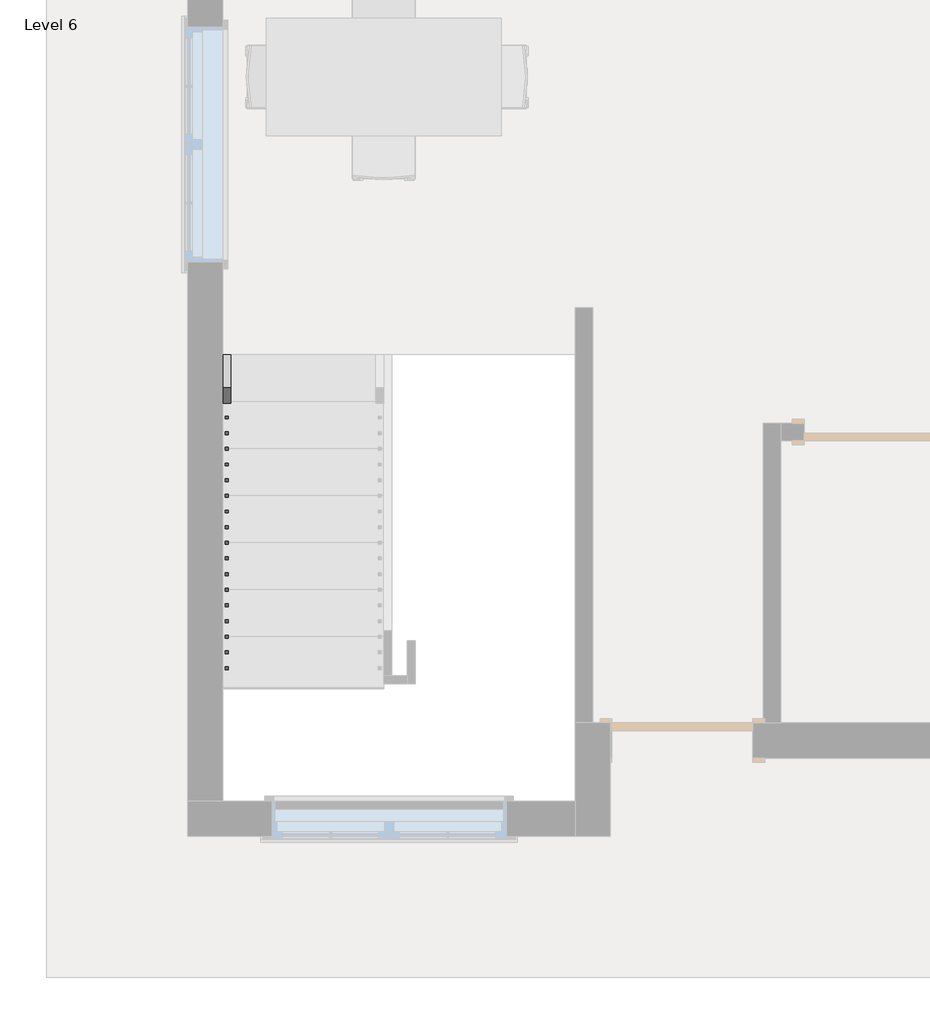
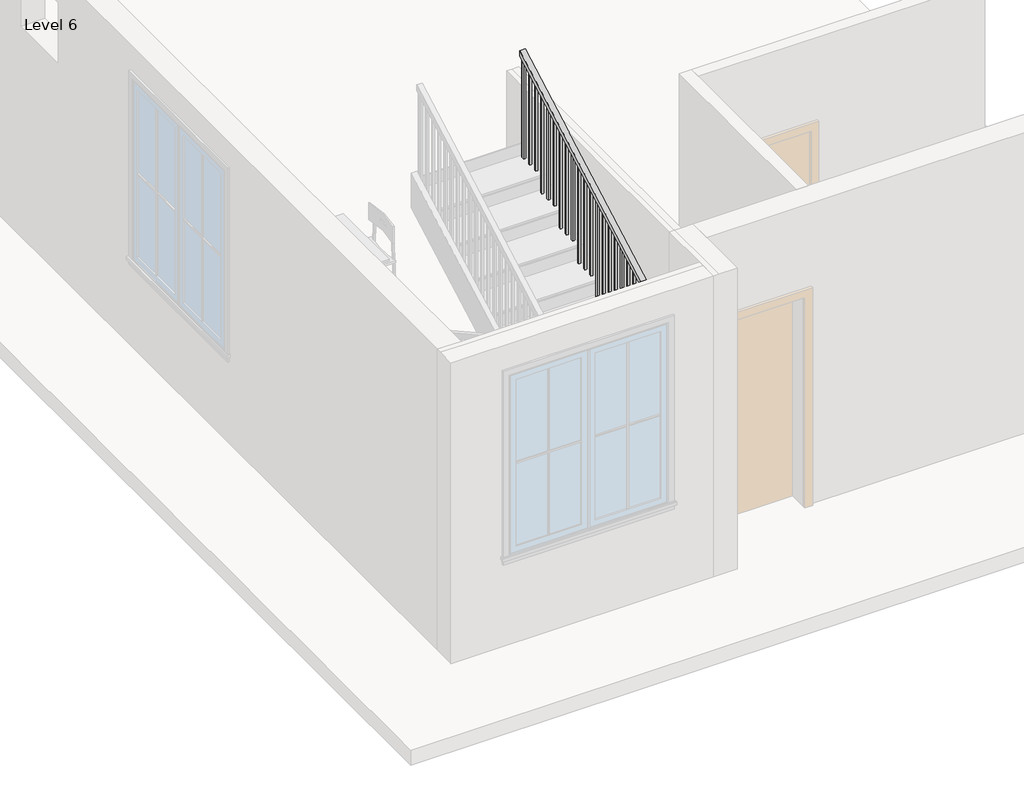
# One storey, part 2 of 3: 1 railing.
"""IFC4 building model written with IfcOpenShell, lengths in millimetres."""

from ifc_helpers import new_model, si_unit, frame, origin, place, context, project, spatial, polyline, outline, extrude, faceted_brep, element, save

model = new_model("IFC4")

# Units and contexts
model_context = context("Model", 3, world=origin())
ifc_project = project(units=[si_unit("LENGTHUNIT", "METRE", prefix="MILLI")], contexts=[model_context])

# Site, building, storey
site = spatial("IfcSite", under=ifc_project)
building = spatial("IfcBuilding", under=site)
storey = spatial("IfcBuildingStorey", under=building, Name="Level 6", Elevation=15849.6)

# Railing
placement = place(None, origin())
element("IfcRailing", 1, ObjectType="Handrail - Rectangular", at=placement, inside=storey, context=model_context, shape_type="SolidModel", body=[
    faceted_brep([(-4181.480864, -3571.6080018, 16933.3333333), (-4181.480864, -3571.6080018, 16875.220221), (-4232.280864, -3571.6080018, 16875.220221), (-4232.280864, -3571.6080018, 16933.3333333), (-4181.480864, -5705.2080018, 18118.6666667), (-4181.480864, -5718.371604, 18067.8666667), (-4232.280864, -5718.371604, 18067.8666667), (-4232.280864, -5705.2080018, 18118.6666667), (-4181.480864, -6416.4080018, 18118.6666667), (-4181.480864, -6416.4080018, 18067.8666667), (-4232.280864, -6467.2080018, 18067.8666667), (-4232.280864, -6467.2080018, 18118.6666667), (-1997.080864, -6416.4080018, 18118.6666667), (-1997.080864, -6416.4080018, 18067.8666667), (-1946.280864, -6467.2080018, 18067.8666667), (-1946.280864, -6467.2080018, 18118.6666667), (-1997.080864, -5705.2080018, 18118.6666667), (-1997.080864, -5692.0443995, 18067.8666667), (-1946.280864, -5692.0443995, 18067.8666667), (-1946.280864, -5705.2080018, 18118.6666667), (-1997.080864, -3571.6080018, 19304.0), (-1946.280864, -3571.6080018, 19304.0), (-1946.280864, -3571.6080018, 19245.8868876), (-1997.080864, -3571.6080018, 19245.8868876)], [[[0, 1, 2, 3]], [[1, 0, 4, 5]], [[2, 1, 5, 6]], [[3, 2, 6, 7]], [[0, 3, 7, 4]], [[5, 4, 8, 9]], [[6, 5, 9, 10]], [[7, 6, 10, 11]], [[4, 7, 11, 8]], [[9, 8, 12, 13]], [[10, 9, 13, 14]], [[11, 10, 14, 15]], [[8, 11, 15, 12]], [[13, 12, 16, 17]], [[14, 13, 17, 18]], [[15, 14, 18, 19]], [[12, 15, 19, 16]], [[20, 21, 22, 23]], [[17, 16, 20, 23]], [[18, 17, 23, 22]], [[19, 18, 22, 21]], [[16, 19, 21, 20]]]),
    extrude(outline(polyline([(-3606.5330018, 19226.4841099), (-3587.4830018, 19237.0674432), (-3587.4830018, 18220.2666667), (-3606.5330018, 18220.2666667), (-3606.5330018, 19226.4841099)])), frame((-1981.205864, 0.0, 0.0), z_axis=(1.0, 0.0, 0.0), x_axis=(0.0, 1.0, 0.0)), (0.0, 0.0, 1.0), 19.05),
    extrude(outline(polyline([(-3708.1330018, 19170.0396654), (-3689.0830018, 19180.6229988), (-3689.0830018, 18220.2666667), (-3708.1330018, 18220.2666667), (-3708.1330018, 19170.0396654)])), frame((-1981.205864, 0.0, 0.0), z_axis=(1.0, 0.0, 0.0), x_axis=(0.0, 1.0, 0.0)), (0.0, 0.0, 1.0), 19.05),
    extrude(outline(polyline([(-3809.7330018, 19113.595221), (-3790.6830018, 19124.1785543), (-3790.6830018, 18220.2666667), (-3809.7330018, 18220.2666667), (-3809.7330018, 19113.595221)])), frame((-1981.205864, 0.0, 0.0), z_axis=(1.0, 0.0, 0.0), x_axis=(0.0, 1.0, 0.0)), (0.0, 0.0, 1.0), 19.05),
    extrude(outline(polyline([(-3911.3330018, 19057.1507765), (-3892.2830018, 19067.7341099), (-3892.2830018, 18050.9333333), (-3911.3330018, 18050.9333333), (-3911.3330018, 19057.1507765)])), frame((-1981.205864, 0.0, 0.0), z_axis=(1.0, 0.0, 0.0), x_axis=(0.0, 1.0, 0.0)), (0.0, 0.0, 1.0), 19.05),
    extrude(outline(polyline([(-4012.9330018, 19000.7063321), (-3993.8830018, 19011.2896654), (-3993.8830018, 18050.9333333), (-4012.9330018, 18050.9333333), (-4012.9330018, 19000.7063321)])), frame((-1981.205864, 0.0, 0.0), z_axis=(1.0, 0.0, 0.0), x_axis=(0.0, 1.0, 0.0)), (0.0, 0.0, 1.0), 19.05),
    extrude(outline(polyline([(-4114.5330018, 18944.2618876), (-4095.4830018, 18954.845221), (-4095.4830018, 18050.9333333), (-4114.5330018, 18050.9333333), (-4114.5330018, 18944.2618876)])), frame((-1981.205864, 0.0, 0.0), z_axis=(1.0, 0.0, 0.0), x_axis=(0.0, 1.0, 0.0)), (0.0, 0.0, 1.0), 19.05),
    extrude(outline(polyline([(-4216.1330018, 18887.8174432), (-4197.0830018, 18898.4007765), (-4197.0830018, 17881.6), (-4216.1330018, 17881.6), (-4216.1330018, 18887.8174432)])), frame((-1981.205864, 0.0, 0.0), z_axis=(1.0, 0.0, 0.0), x_axis=(0.0, 1.0, 0.0)), (0.0, 0.0, 1.0), 19.05),
    extrude(outline(polyline([(-4317.7330018, 18831.3729988), (-4298.6830018, 18841.9563321), (-4298.6830018, 17881.6), (-4317.7330018, 17881.6), (-4317.7330018, 18831.3729988)])), frame((-1981.205864, 0.0, 0.0), z_axis=(1.0, 0.0, 0.0), x_axis=(0.0, 1.0, 0.0)), (0.0, 0.0, 1.0), 19.05),
    extrude(outline(polyline([(-4419.3330018, 18774.9285543), (-4400.2830018, 18785.5118876), (-4400.2830018, 17881.6), (-4419.3330018, 17881.6), (-4419.3330018, 18774.9285543)])), frame((-1981.205864, 0.0, 0.0), z_axis=(1.0, 0.0, 0.0), x_axis=(0.0, 1.0, 0.0)), (0.0, 0.0, 1.0), 19.05),
    extrude(outline(polyline([(-4520.9330018, 18718.4841099), (-4501.8830018, 18729.0674432), (-4501.8830018, 17712.2666667), (-4520.9330018, 17712.2666667), (-4520.9330018, 18718.4841099)])), frame((-1981.205864, 0.0, 0.0), z_axis=(1.0, 0.0, 0.0), x_axis=(0.0, 1.0, 0.0)), (0.0, 0.0, 1.0), 19.05),
    extrude(outline(polyline([(-4622.5330018, 18662.0396654), (-4603.4830018, 18672.6229988), (-4603.4830018, 17712.2666667), (-4622.5330018, 17712.2666667), (-4622.5330018, 18662.0396654)])), frame((-1981.205864, 0.0, 0.0), z_axis=(1.0, 0.0, 0.0), x_axis=(0.0, 1.0, 0.0)), (0.0, 0.0, 1.0), 19.05),
    extrude(outline(polyline([(-4724.1330018, 18605.595221), (-4705.0830018, 18616.1785543), (-4705.0830018, 17712.2666667), (-4724.1330018, 17712.2666667), (-4724.1330018, 18605.595221)])), frame((-1981.205864, 0.0, 0.0), z_axis=(1.0, 0.0, 0.0), x_axis=(0.0, 1.0, 0.0)), (0.0, 0.0, 1.0), 19.05),
    extrude(outline(polyline([(-4825.7330018, 18549.1507765), (-4806.6830018, 18559.7341099), (-4806.6830018, 17542.9333333), (-4825.7330018, 17542.9333333), (-4825.7330018, 18549.1507765)])), frame((-1981.205864, 0.0, 0.0), z_axis=(1.0, 0.0, 0.0), x_axis=(0.0, 1.0, 0.0)), (0.0, 0.0, 1.0), 19.05),
    extrude(outline(polyline([(-4927.3330018, 18492.7063321), (-4908.2830018, 18503.2896654), (-4908.2830018, 17542.9333333), (-4927.3330018, 17542.9333333), (-4927.3330018, 18492.7063321)])), frame((-1981.205864, 0.0, 0.0), z_axis=(1.0, 0.0, 0.0), x_axis=(0.0, 1.0, 0.0)), (0.0, 0.0, 1.0), 19.05),
    extrude(outline(polyline([(-5028.9330018, 18436.2618876), (-5009.8830018, 18446.845221), (-5009.8830018, 17542.9333333), (-5028.9330018, 17542.9333333), (-5028.9330018, 18436.2618876)])), frame((-1981.205864, 0.0, 0.0), z_axis=(1.0, 0.0, 0.0), x_axis=(0.0, 1.0, 0.0)), (0.0, 0.0, 1.0), 19.05),
    extrude(outline(polyline([(-5130.5330018, 18379.8174432), (-5111.4830018, 18390.4007765), (-5111.4830018, 17373.6), (-5130.5330018, 17373.6), (-5130.5330018, 18379.8174432)])), frame((-1981.205864, 0.0, 0.0), z_axis=(1.0, 0.0, 0.0), x_axis=(0.0, 1.0, 0.0)), (0.0, 0.0, 1.0), 19.05),
    extrude(outline(polyline([(-5232.1330018, 18323.3729988), (-5213.0830018, 18333.9563321), (-5213.0830018, 17373.6), (-5232.1330018, 17373.6), (-5232.1330018, 18323.3729988)])), frame((-1981.205864, 0.0, 0.0), z_axis=(1.0, 0.0, 0.0), x_axis=(0.0, 1.0, 0.0)), (0.0, 0.0, 1.0), 19.05),
    extrude(outline(polyline([(-5333.7330018, 18266.9285543), (-5314.6830018, 18277.5118876), (-5314.6830018, 17373.6), (-5333.7330018, 17373.6), (-5333.7330018, 18266.9285543)])), frame((-1981.205864, 0.0, 0.0), z_axis=(1.0, 0.0, 0.0), x_axis=(0.0, 1.0, 0.0)), (0.0, 0.0, 1.0), 19.05),
    extrude(outline(polyline([(-5435.3330018, 18210.4841099), (-5416.2830018, 18221.0674432), (-5416.2830018, 17204.2666667), (-5435.3330018, 17204.2666667), (-5435.3330018, 18210.4841099)])), frame((-1981.205864, 0.0, 0.0), z_axis=(1.0, 0.0, 0.0), x_axis=(0.0, 1.0, 0.0)), (0.0, 0.0, 1.0), 19.05),
    extrude(outline(polyline([(-5536.9330018, 18154.0396654), (-5517.8830018, 18164.6229988), (-5517.8830018, 17204.2666667), (-5536.9330018, 17204.2666667), (-5536.9330018, 18154.0396654)])), frame((-1981.205864, 0.0, 0.0), z_axis=(1.0, 0.0, 0.0), x_axis=(0.0, 1.0, 0.0)), (0.0, 0.0, 1.0), 19.05),
    extrude(outline(polyline([(-5638.5330018, 18097.595221), (-5619.4830018, 18108.1785543), (-5619.4830018, 17204.2666667), (-5638.5330018, 17204.2666667), (-5638.5330018, 18097.595221)])), frame((-1981.205864, 0.0, 0.0), z_axis=(1.0, 0.0, 0.0), x_axis=(0.0, 1.0, 0.0)), (0.0, 0.0, 1.0), 19.05),
    extrude(outline(polyline([(-1962.155864, -5740.1330018), (-1981.205864, -5740.1330018), (-1981.205864, -5721.0830018), (-1962.155864, -5721.0830018), (-1962.155864, -5740.1330018)])), frame((0.0, 0.0, 17204.2666667), z_axis=(0.0, 0.0, 1.0), x_axis=(1.0, 0.0, 0.0)), (0.0, 0.0, 1.0), 863.6),
    extrude(outline(polyline([(-1962.155864, -5841.7330018), (-1981.205864, -5841.7330018), (-1981.205864, -5822.6830018), (-1962.155864, -5822.6830018), (-1962.155864, -5841.7330018)])), frame((0.0, 0.0, 17204.2666667), z_axis=(0.0, 0.0, 1.0), x_axis=(1.0, 0.0, 0.0)), (0.0, 0.0, 1.0), 863.6),
    extrude(outline(polyline([(-1962.155864, -5943.3330018), (-1981.205864, -5943.3330018), (-1981.205864, -5924.2830018), (-1962.155864, -5924.2830018), (-1962.155864, -5943.3330018)])), frame((0.0, 0.0, 17204.2666667), z_axis=(0.0, 0.0, 1.0), x_axis=(1.0, 0.0, 0.0)), (0.0, 0.0, 1.0), 863.6),
    extrude(outline(polyline([(-1962.155864, -6044.9330018), (-1981.205864, -6044.9330018), (-1981.205864, -6025.8830018), (-1962.155864, -6025.8830018), (-1962.155864, -6044.9330018)])), frame((0.0, 0.0, 17204.2666667), z_axis=(0.0, 0.0, 1.0), x_axis=(1.0, 0.0, 0.0)), (0.0, 0.0, 1.0), 863.6),
    extrude(outline(polyline([(-1962.155864, -6146.5330018), (-1981.205864, -6146.5330018), (-1981.205864, -6127.4830018), (-1962.155864, -6127.4830018), (-1962.155864, -6146.5330018)])), frame((0.0, 0.0, 17204.2666667), z_axis=(0.0, 0.0, 1.0), x_axis=(1.0, 0.0, 0.0)), (0.0, 0.0, 1.0), 863.6),
    extrude(outline(polyline([(-1962.155864, -6248.1330018), (-1981.205864, -6248.1330018), (-1981.205864, -6229.0830018), (-1962.155864, -6229.0830018), (-1962.155864, -6248.1330018)])), frame((0.0, 0.0, 17204.2666667), z_axis=(0.0, 0.0, 1.0), x_axis=(1.0, 0.0, 0.0)), (0.0, 0.0, 1.0), 863.6),
    extrude(outline(polyline([(-1962.155864, -6349.7330018), (-1981.205864, -6349.7330018), (-1981.205864, -6330.6830018), (-1962.155864, -6330.6830018), (-1962.155864, -6349.7330018)])), frame((0.0, 0.0, 17204.2666667), z_axis=(0.0, 0.0, 1.0), x_axis=(1.0, 0.0, 0.0)), (0.0, 0.0, 1.0), 863.6),
    extrude(outline(polyline([(-2082.805864, -6451.3330018), (-2082.805864, -6432.2830018), (-2063.755864, -6432.2830018), (-2063.755864, -6451.3330018), (-2082.805864, -6451.3330018)])), frame((0.0, 0.0, 17204.2666667), z_axis=(0.0, 0.0, 1.0), x_axis=(1.0, 0.0, 0.0)), (0.0, 0.0, 1.0), 863.6),
    extrude(outline(polyline([(-2184.405864, -6451.3330018), (-2184.405864, -6432.2830018), (-2165.355864, -6432.2830018), (-2165.355864, -6451.3330018), (-2184.405864, -6451.3330018)])), frame((0.0, 0.0, 17204.2666667), z_axis=(0.0, 0.0, 1.0), x_axis=(1.0, 0.0, 0.0)), (0.0, 0.0, 1.0), 863.6),
    extrude(outline(polyline([(-2286.005864, -6451.3330018), (-2286.005864, -6432.2830018), (-2266.955864, -6432.2830018), (-2266.955864, -6451.3330018), (-2286.005864, -6451.3330018)])), frame((0.0, 0.0, 17204.2666667), z_axis=(0.0, 0.0, 1.0), x_axis=(1.0, 0.0, 0.0)), (0.0, 0.0, 1.0), 863.6),
    extrude(outline(polyline([(-2387.605864, -6451.3330018), (-2387.605864, -6432.2830018), (-2368.555864, -6432.2830018), (-2368.555864, -6451.3330018), (-2387.605864, -6451.3330018)])), frame((0.0, 0.0, 17204.2666667), z_axis=(0.0, 0.0, 1.0), x_axis=(1.0, 0.0, 0.0)), (0.0, 0.0, 1.0), 863.6),
    extrude(outline(polyline([(-2489.205864, -6451.3330018), (-2489.205864, -6432.2830018), (-2470.155864, -6432.2830018), (-2470.155864, -6451.3330018), (-2489.205864, -6451.3330018)])), frame((0.0, 0.0, 17204.2666667), z_axis=(0.0, 0.0, 1.0), x_axis=(1.0, 0.0, 0.0)), (0.0, 0.0, 1.0), 863.6),
    extrude(outline(polyline([(-2590.805864, -6451.3330018), (-2590.805864, -6432.2830018), (-2571.755864, -6432.2830018), (-2571.755864, -6451.3330018), (-2590.805864, -6451.3330018)])), frame((0.0, 0.0, 17204.2666667), z_axis=(0.0, 0.0, 1.0), x_axis=(1.0, 0.0, 0.0)), (0.0, 0.0, 1.0), 863.6),
    extrude(outline(polyline([(-2692.405864, -6451.3330018), (-2692.405864, -6432.2830018), (-2673.355864, -6432.2830018), (-2673.355864, -6451.3330018), (-2692.405864, -6451.3330018)])), frame((0.0, 0.0, 17204.2666667), z_axis=(0.0, 0.0, 1.0), x_axis=(1.0, 0.0, 0.0)), (0.0, 0.0, 1.0), 863.6),
    extrude(outline(polyline([(-2794.005864, -6451.3330018), (-2794.005864, -6432.2830018), (-2774.955864, -6432.2830018), (-2774.955864, -6451.3330018), (-2794.005864, -6451.3330018)])), frame((0.0, 0.0, 17204.2666667), z_axis=(0.0, 0.0, 1.0), x_axis=(1.0, 0.0, 0.0)), (0.0, 0.0, 1.0), 863.6),
    extrude(outline(polyline([(-2895.605864, -6451.3330018), (-2895.605864, -6432.2830018), (-2876.555864, -6432.2830018), (-2876.555864, -6451.3330018), (-2895.605864, -6451.3330018)])), frame((0.0, 0.0, 17204.2666667), z_axis=(0.0, 0.0, 1.0), x_axis=(1.0, 0.0, 0.0)), (0.0, 0.0, 1.0), 863.6),
    extrude(outline(polyline([(-2997.205864, -6451.3330018), (-2997.205864, -6432.2830018), (-2978.155864, -6432.2830018), (-2978.155864, -6451.3330018), (-2997.205864, -6451.3330018)])), frame((0.0, 0.0, 17204.2666667), z_axis=(0.0, 0.0, 1.0), x_axis=(1.0, 0.0, 0.0)), (0.0, 0.0, 1.0), 863.6),
    extrude(outline(polyline([(-3098.805864, -6451.3330018), (-3098.805864, -6432.2830018), (-3079.755864, -6432.2830018), (-3079.755864, -6451.3330018), (-3098.805864, -6451.3330018)])), frame((0.0, 0.0, 17204.2666667), z_axis=(0.0, 0.0, 1.0), x_axis=(1.0, 0.0, 0.0)), (0.0, 0.0, 1.0), 863.6),
    extrude(outline(polyline([(-3200.405864, -6451.3330018), (-3200.405864, -6432.2830018), (-3181.355864, -6432.2830018), (-3181.355864, -6451.3330018), (-3200.405864, -6451.3330018)])), frame((0.0, 0.0, 17204.2666667), z_axis=(0.0, 0.0, 1.0), x_axis=(1.0, 0.0, 0.0)), (0.0, 0.0, 1.0), 863.6),
    extrude(outline(polyline([(-3302.005864, -6451.3330018), (-3302.005864, -6432.2830018), (-3282.955864, -6432.2830018), (-3282.955864, -6451.3330018), (-3302.005864, -6451.3330018)])), frame((0.0, 0.0, 17204.2666667), z_axis=(0.0, 0.0, 1.0), x_axis=(1.0, 0.0, 0.0)), (0.0, 0.0, 1.0), 863.6),
    extrude(outline(polyline([(-3403.605864, -6451.3330018), (-3403.605864, -6432.2830018), (-3384.555864, -6432.2830018), (-3384.555864, -6451.3330018), (-3403.605864, -6451.3330018)])), frame((0.0, 0.0, 17204.2666667), z_axis=(0.0, 0.0, 1.0), x_axis=(1.0, 0.0, 0.0)), (0.0, 0.0, 1.0), 863.6),
    extrude(outline(polyline([(-3505.205864, -6451.3330018), (-3505.205864, -6432.2830018), (-3486.155864, -6432.2830018), (-3486.155864, -6451.3330018), (-3505.205864, -6451.3330018)])), frame((0.0, 0.0, 17204.2666667), z_axis=(0.0, 0.0, 1.0), x_axis=(1.0, 0.0, 0.0)), (0.0, 0.0, 1.0), 863.6),
    extrude(outline(polyline([(-3606.805864, -6451.3330018), (-3606.805864, -6432.2830018), (-3587.755864, -6432.2830018), (-3587.755864, -6451.3330018), (-3606.805864, -6451.3330018)])), frame((0.0, 0.0, 17204.2666667), z_axis=(0.0, 0.0, 1.0), x_axis=(1.0, 0.0, 0.0)), (0.0, 0.0, 1.0), 863.6),
    extrude(outline(polyline([(-3708.405864, -6451.3330018), (-3708.405864, -6432.2830018), (-3689.355864, -6432.2830018), (-3689.355864, -6451.3330018), (-3708.405864, -6451.3330018)])), frame((0.0, 0.0, 17204.2666667), z_axis=(0.0, 0.0, 1.0), x_axis=(1.0, 0.0, 0.0)), (0.0, 0.0, 1.0), 863.6),
    extrude(outline(polyline([(-3810.005864, -6451.3330018), (-3810.005864, -6432.2830018), (-3790.955864, -6432.2830018), (-3790.955864, -6451.3330018), (-3810.005864, -6451.3330018)])), frame((0.0, 0.0, 17204.2666667), z_axis=(0.0, 0.0, 1.0), x_axis=(1.0, 0.0, 0.0)), (0.0, 0.0, 1.0), 863.6),
    extrude(outline(polyline([(-3911.605864, -6451.3330018), (-3911.605864, -6432.2830018), (-3892.555864, -6432.2830018), (-3892.555864, -6451.3330018), (-3911.605864, -6451.3330018)])), frame((0.0, 0.0, 17204.2666667), z_axis=(0.0, 0.0, 1.0), x_axis=(1.0, 0.0, 0.0)), (0.0, 0.0, 1.0), 863.6),
    extrude(outline(polyline([(-4013.205864, -6451.3330018), (-4013.205864, -6432.2830018), (-3994.155864, -6432.2830018), (-3994.155864, -6451.3330018), (-4013.205864, -6451.3330018)])), frame((0.0, 0.0, 17204.2666667), z_axis=(0.0, 0.0, 1.0), x_axis=(1.0, 0.0, 0.0)), (0.0, 0.0, 1.0), 863.6),
    extrude(outline(polyline([(-4114.805864, -6451.3330018), (-4114.805864, -6432.2830018), (-4095.755864, -6432.2830018), (-4095.755864, -6451.3330018), (-4114.805864, -6451.3330018)])), frame((0.0, 0.0, 17204.2666667), z_axis=(0.0, 0.0, 1.0), x_axis=(1.0, 0.0, 0.0)), (0.0, 0.0, 1.0), 863.6),
    extrude(outline(polyline([(-4216.405864, -6406.8830018), (-4197.355864, -6406.8830018), (-4197.355864, -6425.9330018), (-4216.405864, -6425.9330018), (-4216.405864, -6406.8830018)])), frame((0.0, 0.0, 17204.2666667), z_axis=(0.0, 0.0, 1.0), x_axis=(1.0, 0.0, 0.0)), (0.0, 0.0, 1.0), 863.6),
    extrude(outline(polyline([(-4216.405864, -6305.2830018), (-4197.355864, -6305.2830018), (-4197.355864, -6324.3330018), (-4216.405864, -6324.3330018), (-4216.405864, -6305.2830018)])), frame((0.0, 0.0, 17204.2666667), z_axis=(0.0, 0.0, 1.0), x_axis=(1.0, 0.0, 0.0)), (0.0, 0.0, 1.0), 863.6),
    extrude(outline(polyline([(-4216.405864, -6203.6830018), (-4197.355864, -6203.6830018), (-4197.355864, -6222.7330018), (-4216.405864, -6222.7330018), (-4216.405864, -6203.6830018)])), frame((0.0, 0.0, 17204.2666667), z_axis=(0.0, 0.0, 1.0), x_axis=(1.0, 0.0, 0.0)), (0.0, 0.0, 1.0), 863.6),
    extrude(outline(polyline([(-4216.405864, -6102.0830018), (-4197.355864, -6102.0830018), (-4197.355864, -6121.1330018), (-4216.405864, -6121.1330018), (-4216.405864, -6102.0830018)])), frame((0.0, 0.0, 17204.2666667), z_axis=(0.0, 0.0, 1.0), x_axis=(1.0, 0.0, 0.0)), (0.0, 0.0, 1.0), 863.6),
    extrude(outline(polyline([(-4216.405864, -6000.4830018), (-4197.355864, -6000.4830018), (-4197.355864, -6019.5330018), (-4216.405864, -6019.5330018), (-4216.405864, -6000.4830018)])), frame((0.0, 0.0, 17204.2666667), z_axis=(0.0, 0.0, 1.0), x_axis=(1.0, 0.0, 0.0)), (0.0, 0.0, 1.0), 863.6),
    extrude(outline(polyline([(-4216.405864, -5898.8830018), (-4197.355864, -5898.8830018), (-4197.355864, -5917.9330018), (-4216.405864, -5917.9330018), (-4216.405864, -5898.8830018)])), frame((0.0, 0.0, 17204.2666667), z_axis=(0.0, 0.0, 1.0), x_axis=(1.0, 0.0, 0.0)), (0.0, 0.0, 1.0), 863.6),
    extrude(outline(polyline([(-4216.405864, -5797.2830018), (-4197.355864, -5797.2830018), (-4197.355864, -5816.3330018), (-4216.405864, -5816.3330018), (-4216.405864, -5797.2830018)])), frame((0.0, 0.0, 17204.2666667), z_axis=(0.0, 0.0, 1.0), x_axis=(1.0, 0.0, 0.0)), (0.0, 0.0, 1.0), 863.6),
    extrude(outline(polyline([(-5714.7330018, 18065.845221), (-5695.6830018, 18055.2618876), (-5695.6830018, 17204.2666667), (-5714.7330018, 17204.2666667), (-5714.7330018, 18065.845221)])), frame((-4216.405864, 0.0, 0.0), z_axis=(1.0, 0.0, 0.0), x_axis=(0.0, 1.0, 0.0)), (0.0, 0.0, 1.0), 19.05),
    extrude(outline(polyline([(-5613.1330018, 18009.4007765), (-5594.0830018, 17998.8174432), (-5594.0830018, 17034.9333333), (-5613.1330018, 17034.9333333), (-5613.1330018, 18009.4007765)])), frame((-4216.405864, 0.0, 0.0), z_axis=(1.0, 0.0, 0.0), x_axis=(0.0, 1.0, 0.0)), (0.0, 0.0, 1.0), 19.05),
    extrude(outline(polyline([(-5511.5330018, 17952.9563321), (-5492.4830018, 17942.3729988), (-5492.4830018, 17034.9333333), (-5511.5330018, 17034.9333333), (-5511.5330018, 17952.9563321)])), frame((-4216.405864, 0.0, 0.0), z_axis=(1.0, 0.0, 0.0), x_axis=(0.0, 1.0, 0.0)), (0.0, 0.0, 1.0), 19.05),
    extrude(outline(polyline([(-5409.9330018, 17896.5118876), (-5390.8830018, 17885.9285543), (-5390.8830018, 17034.9333333), (-5409.9330018, 17034.9333333), (-5409.9330018, 17896.5118876)])), frame((-4216.405864, 0.0, 0.0), z_axis=(1.0, 0.0, 0.0), x_axis=(0.0, 1.0, 0.0)), (0.0, 0.0, 1.0), 19.05),
    extrude(outline(polyline([(-5308.3330018, 17840.0674432), (-5289.2830018, 17829.4841099), (-5289.2830018, 16865.6), (-5308.3330018, 16865.6), (-5308.3330018, 17840.0674432)])), frame((-4216.405864, 0.0, 0.0), z_axis=(1.0, 0.0, 0.0), x_axis=(0.0, 1.0, 0.0)), (0.0, 0.0, 1.0), 19.05),
    extrude(outline(polyline([(-5206.7330018, 17783.6229988), (-5187.6830018, 17773.0396654), (-5187.6830018, 16865.6), (-5206.7330018, 16865.6), (-5206.7330018, 17783.6229988)])), frame((-4216.405864, 0.0, 0.0), z_axis=(1.0, 0.0, 0.0), x_axis=(0.0, 1.0, 0.0)), (0.0, 0.0, 1.0), 19.05),
    extrude(outline(polyline([(-5105.1330018, 17727.1785543), (-5086.0830018, 17716.595221), (-5086.0830018, 16865.6), (-5105.1330018, 16865.6), (-5105.1330018, 17727.1785543)])), frame((-4216.405864, 0.0, 0.0), z_axis=(1.0, 0.0, 0.0), x_axis=(0.0, 1.0, 0.0)), (0.0, 0.0, 1.0), 19.05),
    extrude(outline(polyline([(-5003.5330018, 17670.7341099), (-4984.4830018, 17660.1507765), (-4984.4830018, 16696.2666667), (-5003.5330018, 16696.2666667), (-5003.5330018, 17670.7341099)])), frame((-4216.405864, 0.0, 0.0), z_axis=(1.0, 0.0, 0.0), x_axis=(0.0, 1.0, 0.0)), (0.0, 0.0, 1.0), 19.05),
    extrude(outline(polyline([(-4901.9330018, 17614.2896654), (-4882.8830018, 17603.7063321), (-4882.8830018, 16696.2666667), (-4901.9330018, 16696.2666667), (-4901.9330018, 17614.2896654)])), frame((-4216.405864, 0.0, 0.0), z_axis=(1.0, 0.0, 0.0), x_axis=(0.0, 1.0, 0.0)), (0.0, 0.0, 1.0), 19.05),
    extrude(outline(polyline([(-4800.3330018, 17557.845221), (-4781.2830018, 17547.2618876), (-4781.2830018, 16696.2666667), (-4800.3330018, 16696.2666667), (-4800.3330018, 17557.845221)])), frame((-4216.405864, 0.0, 0.0), z_axis=(1.0, 0.0, 0.0), x_axis=(0.0, 1.0, 0.0)), (0.0, 0.0, 1.0), 19.05),
    extrude(outline(polyline([(-4698.7330018, 17501.4007765), (-4679.6830018, 17490.8174432), (-4679.6830018, 16526.9333333), (-4698.7330018, 16526.9333333), (-4698.7330018, 17501.4007765)])), frame((-4216.405864, 0.0, 0.0), z_axis=(1.0, 0.0, 0.0), x_axis=(0.0, 1.0, 0.0)), (0.0, 0.0, 1.0), 19.05),
    extrude(outline(polyline([(-4597.1330018, 17444.9563321), (-4578.0830018, 17434.3729988), (-4578.0830018, 16526.9333333), (-4597.1330018, 16526.9333333), (-4597.1330018, 17444.9563321)])), frame((-4216.405864, 0.0, 0.0), z_axis=(1.0, 0.0, 0.0), x_axis=(0.0, 1.0, 0.0)), (0.0, 0.0, 1.0), 19.05),
    extrude(outline(polyline([(-4495.5330018, 17388.5118876), (-4476.4830018, 17377.9285543), (-4476.4830018, 16526.9333333), (-4495.5330018, 16526.9333333), (-4495.5330018, 17388.5118876)])), frame((-4216.405864, 0.0, 0.0), z_axis=(1.0, 0.0, 0.0), x_axis=(0.0, 1.0, 0.0)), (0.0, 0.0, 1.0), 19.05),
    extrude(outline(polyline([(-4393.9330018, 17332.0674432), (-4374.8830018, 17321.4841099), (-4374.8830018, 16357.6), (-4393.9330018, 16357.6), (-4393.9330018, 17332.0674432)])), frame((-4216.405864, 0.0, 0.0), z_axis=(1.0, 0.0, 0.0), x_axis=(0.0, 1.0, 0.0)), (0.0, 0.0, 1.0), 19.05),
    extrude(outline(polyline([(-4292.3330018, 17275.6229988), (-4273.2830018, 17265.0396654), (-4273.2830018, 16357.6), (-4292.3330018, 16357.6), (-4292.3330018, 17275.6229988)])), frame((-4216.405864, 0.0, 0.0), z_axis=(1.0, 0.0, 0.0), x_axis=(0.0, 1.0, 0.0)), (0.0, 0.0, 1.0), 19.05),
    extrude(outline(polyline([(-4190.7330018, 17219.1785543), (-4171.6830018, 17208.595221), (-4171.6830018, 16357.6), (-4190.7330018, 16357.6), (-4190.7330018, 17219.1785543)])), frame((-4216.405864, 0.0, 0.0), z_axis=(1.0, 0.0, 0.0), x_axis=(0.0, 1.0, 0.0)), (0.0, 0.0, 1.0), 19.05),
    extrude(outline(polyline([(-4089.1330018, 17162.7341099), (-4070.0830018, 17152.1507765), (-4070.0830018, 16188.2666667), (-4089.1330018, 16188.2666667), (-4089.1330018, 17162.7341099)])), frame((-4216.405864, 0.0, 0.0), z_axis=(1.0, 0.0, 0.0), x_axis=(0.0, 1.0, 0.0)), (0.0, 0.0, 1.0), 19.05),
    extrude(outline(polyline([(-3987.5330018, 17106.2896654), (-3968.4830018, 17095.7063321), (-3968.4830018, 16188.2666667), (-3987.5330018, 16188.2666667), (-3987.5330018, 17106.2896654)])), frame((-4216.405864, 0.0, 0.0), z_axis=(1.0, 0.0, 0.0), x_axis=(0.0, 1.0, 0.0)), (0.0, 0.0, 1.0), 19.05),
    extrude(outline(polyline([(-3885.9330018, 17049.845221), (-3866.8830018, 17039.2618876), (-3866.8830018, 16188.2666667), (-3885.9330018, 16188.2666667), (-3885.9330018, 17049.845221)])), frame((-4216.405864, 0.0, 0.0), z_axis=(1.0, 0.0, 0.0), x_axis=(0.0, 1.0, 0.0)), (0.0, 0.0, 1.0), 19.05),
    extrude(outline(polyline([(-3784.3330018, 16993.4007765), (-3765.2830018, 16982.8174432), (-3765.2830018, 16018.9333333), (-3784.3330018, 16018.9333333), (-3784.3330018, 16993.4007765)])), frame((-4216.405864, 0.0, 0.0), z_axis=(1.0, 0.0, 0.0), x_axis=(0.0, 1.0, 0.0)), (0.0, 0.0, 1.0), 19.05),
    extrude(outline(polyline([(-3682.7330018, 16936.9563321), (-3663.6830018, 16926.3729988), (-3663.6830018, 16018.9333333), (-3682.7330018, 16018.9333333), (-3682.7330018, 16936.9563321)])), frame((-4216.405864, 0.0, 0.0), z_axis=(1.0, 0.0, 0.0), x_axis=(0.0, 1.0, 0.0)), (0.0, 0.0, 1.0), 19.05),
    extrude(outline(polyline([(-1981.205864, -6451.3330018), (-1981.205864, -6432.2830018), (-1962.155864, -6432.2830018), (-1962.155864, -6451.3330018), (-1981.205864, -6451.3330018)])), frame((0.0, 0.0, 17204.2666667), z_axis=(0.0, 0.0, 1.0), x_axis=(1.0, 0.0, 0.0)), (0.0, 0.0, 1.0), 863.6),
    extrude(outline(polyline([(-4216.405864, -6432.2830018), (-4197.355864, -6432.2830018), (-4197.355864, -6451.3330018), (-4216.405864, -6451.3330018), (-4216.405864, -6432.2830018)])), frame((0.0, 0.0, 17204.2666667), z_axis=(0.0, 0.0, 1.0), x_axis=(1.0, 0.0, 0.0)), (0.0, 0.0, 1.0), 863.6),
    extrude(outline(polyline([(-3590.6580018, 19235.3035543), (-3571.6080018, 19245.8868876), (-3571.6080018, 18220.2666667), (-3590.6580018, 18220.2666667), (-3590.6580018, 19235.3035543)])), frame((-1981.205864, 0.0, 0.0), z_axis=(1.0, 0.0, 0.0), x_axis=(0.0, 1.0, 0.0)), (0.0, 0.0, 1.0), 19.05),
    extrude(outline(polyline([(-3590.6580018, 16885.8035543), (-3571.6080018, 16875.220221), (-3571.6080018, 16018.9333333), (-3590.6580018, 16018.9333333), (-3590.6580018, 16885.8035543)])), frame((-4216.405864, 0.0, 0.0), z_axis=(1.0, 0.0, 0.0), x_axis=(0.0, 1.0, 0.0)), (0.0, 0.0, 1.0), 19.05),
])

save(model, "model.ifc")

# Revit data of these elements
# Type "Handrail - Rectangular"
#   Assembly Code = "C2010400"
#   built-in parameter 1008612 = 0.0416667 (stored number, unit not read)
#   built-in parameter 1008611 = 0.0416667 (stored number, unit not read)
#   built-in parameter 1008609 = 0.333333 (stored number, unit not read)
#   built-in parameter 1008604 = 0.166667 (stored number, unit not read)
#   built-in parameter 1008603 = 0.166667 (stored number, unit not read)
#   Railing Height = 3' - 0"
#   built-in parameter 1008630 = 2
#   built-in parameter 1008610 = 2
#   built-in parameter 1008618 = Baluster - Square : 3/4"
# Element 1 (IfcRailing, "Handrail - Rectangular")
#   Phase Created = New Construction
